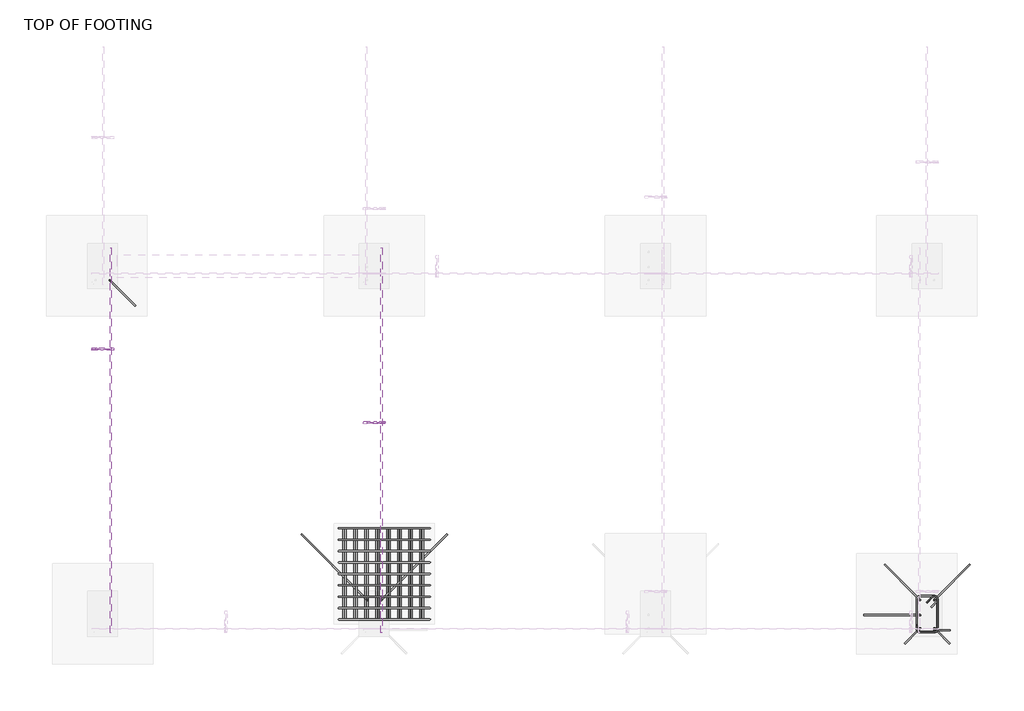
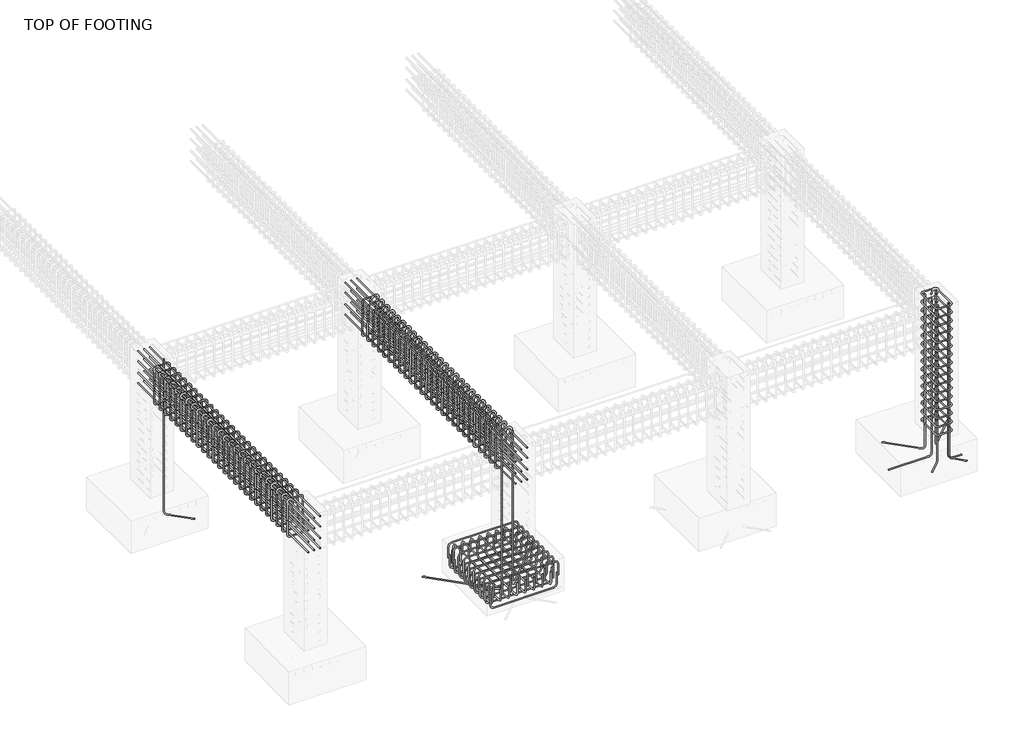
# One storey, part 4 of 14: 24 reinforcing bars.
"""IFC4 building model written with IfcOpenShell, lengths in millimetres."""

from ifc_helpers import new_model, si_unit, point, frame, origin, place, context, project, spatial, polyline, circle_curve, trimmed, segment, composite_curve, source, transform, mapped, element, save
from ifc_brep_helpers import swept_disk

model = new_model("IFC4")

# Units and contexts
model_context = context("Model", 3, world=origin())
ifc_project = project(units=[si_unit("LENGTHUNIT", "METRE", prefix="MILLI")], contexts=[model_context])

# Site, building, storey
site = spatial("IfcSite", under=ifc_project)
building = spatial("IfcBuilding", under=site)
storey = spatial("IfcBuildingStorey", under=building, Name="TOP OF FOOTING", Elevation=-1828.8)

# Reinforcing bars
placement = place(None, origin())
reinforcing_bar_shape = source(origin(), model_context, "Body", "SolidModel", [
    swept_disk(composite_curve([segment(polyline([(-227.457813, 517.7803241, -2035.6107622), (-227.457813, 517.7803241, -2182.9107622)]), True, "CONTINUOUS"), segment(trimmed(circle_curve(frame((-273.807813, 517.7803241, -2182.9107622), z_axis=(0.0, 1.0, 0.0), x_axis=(46.35000000000002, 0.0, 0.0)), 46.35), [point((-227.457813, 517.7803241, -2182.9107622))], [point((-273.807813, 517.7803241, -2229.2607622))], True, "CARTESIAN"), True, "CONTINUOUS"), segment(polyline([(-273.807813, 517.7803241, -2229.2607622), (-1046.4382016, 517.7803241, -2229.2607622)]), True, "CONTINUOUS"), segment(trimmed(circle_curve(frame((-1046.4382016, 517.7803241, -2182.9107622), z_axis=(0.0, 1.0, 0.0), x_axis=(0.0, 0.0, -46.34999999999991)), 46.35), [point((-1046.4382016, 517.7803241, -2229.2607622))], [point((-1092.7882016, 517.7803241, -2182.9107622))], True, "CARTESIAN"), True, "CONTINUOUS"), segment(polyline([(-1092.7882016, 517.7803241, -2182.9107622), (-1092.7882016, 517.7803241, -2035.6107622)]), True, "CONTINUOUS")], self_intersect=False), 6.35),
])
element("IfcReinforcingBar", 1, at=placement, inside=storey, context=model_context, shape_type="MappedRepresentation", body=[
    mapped(reinforcing_bar_shape, transform((0.0, 0.0, 0.0), x_axis=(1.0, 0.0, 0.0), y_axis=(0.0, 1.0, 0.0), z_axis=(0.0, 0.0, 1.0))),
    mapped(reinforcing_bar_shape, transform((0.0, -113.4125, 0.0), x_axis=(1.0, 0.0, 0.0), y_axis=(0.0, 1.0, 0.0), z_axis=(0.0, 0.0, 1.0))),
    mapped(reinforcing_bar_shape, transform((0.0, -226.825, 0.0), x_axis=(1.0, 0.0, 0.0), y_axis=(0.0, 1.0, 0.0), z_axis=(0.0, 0.0, 1.0))),
    mapped(reinforcing_bar_shape, transform((0.0, -340.2375, 0.0), x_axis=(1.0, 0.0, 0.0), y_axis=(0.0, 1.0, 0.0), z_axis=(0.0, 0.0, 1.0))),
    mapped(reinforcing_bar_shape, transform((0.0, -453.65, 0.0), x_axis=(1.0, 0.0, 0.0), y_axis=(0.0, 1.0, 0.0), z_axis=(0.0, 0.0, 1.0))),
    mapped(reinforcing_bar_shape, transform((0.0, -567.0625, 0.0), x_axis=(1.0, 0.0, 0.0), y_axis=(0.0, 1.0, 0.0), z_axis=(0.0, 0.0, 1.0))),
    mapped(reinforcing_bar_shape, transform((0.0, -680.475, 0.0), x_axis=(1.0, 0.0, 0.0), y_axis=(0.0, 1.0, 0.0), z_axis=(0.0, 0.0, 1.0))),
    mapped(reinforcing_bar_shape, transform((0.0, -793.8875, 0.0), x_axis=(1.0, 0.0, 0.0), y_axis=(0.0, 1.0, 0.0), z_axis=(0.0, 0.0, 1.0))),
    mapped(reinforcing_bar_shape, transform((0.0, -907.3, 0.0), x_axis=(1.0, 0.0, 0.0), y_axis=(0.0, 1.0, 0.0), z_axis=(0.0, 0.0, 1.0))),
])
reinforcing_bar_2_shape = source(origin(), model_context, "Body", "SolidModel", [
    swept_disk(composite_curve([segment(polyline([(-1111.0033787, 517.7803241, -2068.991024), (-1111.0033787, 517.7803241, -1921.691024)]), True, "CONTINUOUS"), segment(trimmed(circle_curve(frame((-1064.6533787, 517.7803241, -1921.691024), z_axis=(0.0, 1.0, 0.0), x_axis=(-46.34999999999991, 0.0, 0.0)), 46.35), [point((-1111.0033787, 517.7803241, -1921.691024))], [point((-1064.6533787, 517.7803241, -1875.341024))], True, "CARTESIAN"), True, "CONTINUOUS"), segment(polyline([(-1064.6533787, 517.7803241, -1875.341024), (-250.0533787, 517.7803241, -1875.341024)]), True, "CONTINUOUS"), segment(trimmed(circle_curve(frame((-250.0533787, 517.7803241, -1921.691024), z_axis=(0.0, 1.0, 0.0), x_axis=(0.0, 0.0, 46.34999999999991)), 46.35), [point((-250.0533787, 517.7803241, -1875.341024))], [point((-203.7033787, 517.7803241, -1921.691024))], True, "CARTESIAN"), True, "CONTINUOUS"), segment(polyline([(-203.7033787, 517.7803241, -1921.691024), (-203.7033787, 517.7803241, -2068.991024)]), True, "CONTINUOUS")], self_intersect=False), 6.35),
])
element("IfcReinforcingBar", 2, at=placement, inside=storey, context=model_context, shape_type="MappedRepresentation", body=[
    mapped(reinforcing_bar_2_shape, transform((0.0, 0.0, 0.0), x_axis=(1.0, 0.0, 0.0), y_axis=(0.0, 1.0, 0.0), z_axis=(0.0, 0.0, 1.0))),
    mapped(reinforcing_bar_2_shape, transform((0.0, -113.4125, 0.0), x_axis=(1.0, 0.0, 0.0), y_axis=(0.0, 1.0, 0.0), z_axis=(0.0, 0.0, 1.0))),
    mapped(reinforcing_bar_2_shape, transform((0.0, -226.825, 0.0), x_axis=(1.0, 0.0, 0.0), y_axis=(0.0, 1.0, 0.0), z_axis=(0.0, 0.0, 1.0))),
    mapped(reinforcing_bar_2_shape, transform((0.0, -340.2375, 0.0), x_axis=(1.0, 0.0, 0.0), y_axis=(0.0, 1.0, 0.0), z_axis=(0.0, 0.0, 1.0))),
    mapped(reinforcing_bar_2_shape, transform((0.0, -453.65, 0.0), x_axis=(1.0, 0.0, 0.0), y_axis=(0.0, 1.0, 0.0), z_axis=(0.0, 0.0, 1.0))),
    mapped(reinforcing_bar_2_shape, transform((0.0, -567.0625, 0.0), x_axis=(1.0, 0.0, 0.0), y_axis=(0.0, 1.0, 0.0), z_axis=(0.0, 0.0, 1.0))),
    mapped(reinforcing_bar_2_shape, transform((0.0, -680.475, 0.0), x_axis=(1.0, 0.0, 0.0), y_axis=(0.0, 1.0, 0.0), z_axis=(0.0, 0.0, 1.0))),
    mapped(reinforcing_bar_2_shape, transform((0.0, -793.8875, 0.0), x_axis=(1.0, 0.0, 0.0), y_axis=(0.0, 1.0, 0.0), z_axis=(0.0, 0.0, 1.0))),
    mapped(reinforcing_bar_2_shape, transform((0.0, -907.3, 0.0), x_axis=(1.0, 0.0, 0.0), y_axis=(0.0, 1.0, 0.0), z_axis=(0.0, 0.0, 1.0))),
])
reinforcing_bar_3_shape = source(origin(), model_context, "Body", "SolidModel", [
    swept_disk(composite_curve([segment(polyline([(-273.4932847, 517.7803241, -2085.4684936), (-273.4932847, 517.7803241, -1938.1684936)]), True, "CONTINUOUS"), segment(trimmed(circle_curve(frame((-273.4932847, 471.4303241, -1938.1684936), z_axis=(1.0, 0.0, 0.0), x_axis=(0.0, 46.35000000000002, 0.0)), 46.35), [point((-273.4932847, 517.7803241, -1938.1684936))], [point((-273.4932847, 471.4303241, -1891.8184936))], True, "CARTESIAN"), True, "CONTINUOUS"), segment(polyline([(-273.4932847, 471.4303241, -1891.8184936), (-273.4932847, -343.1696759, -1891.8184936)]), True, "CONTINUOUS"), segment(trimmed(circle_curve(frame((-273.4932847, -343.1696759, -1938.1684936), z_axis=(1.0, 0.0, 0.0), x_axis=(0.0, 0.0, 46.34999999999991)), 46.35), [point((-273.4932847, -343.1696759, -1891.8184936))], [point((-273.4932847, -389.5196759, -1938.1684936))], True, "CARTESIAN"), True, "CONTINUOUS"), segment(polyline([(-273.4932847, -389.5196759, -1938.1684936), (-273.4932847, -389.5196759, -2085.4684936)]), True, "CONTINUOUS")], self_intersect=False), 6.35),
])
element("IfcReinforcingBar", 3, at=placement, inside=storey, context=model_context, shape_type="MappedRepresentation", body=[
    mapped(reinforcing_bar_3_shape, transform((0.0, 0.0, 0.0), x_axis=(1.0, 0.0, 0.0), y_axis=(0.0, 1.0, 0.0), z_axis=(0.0, 0.0, 1.0))),
    mapped(reinforcing_bar_3_shape, transform((-110.0713853, 0.0, 0.0), x_axis=(1.0, 0.0, 0.0), y_axis=(0.0, 1.0, 0.0), z_axis=(0.0, 0.0, 1.0))),
    mapped(reinforcing_bar_3_shape, transform((-220.1427706, 0.0, 0.0), x_axis=(1.0, 0.0, 0.0), y_axis=(0.0, 1.0, 0.0), z_axis=(0.0, 0.0, 1.0))),
    mapped(reinforcing_bar_3_shape, transform((-330.2141558, 0.0, 0.0), x_axis=(1.0, 0.0, 0.0), y_axis=(0.0, 1.0, 0.0), z_axis=(0.0, 0.0, 1.0))),
    mapped(reinforcing_bar_3_shape, transform((-440.2855411, 0.0, 0.0), x_axis=(1.0, 0.0, 0.0), y_axis=(0.0, 1.0, 0.0), z_axis=(0.0, 0.0, 1.0))),
    mapped(reinforcing_bar_3_shape, transform((-550.3569264, 0.0, 0.0), x_axis=(1.0, 0.0, 0.0), y_axis=(0.0, 1.0, 0.0), z_axis=(0.0, 0.0, 1.0))),
    mapped(reinforcing_bar_3_shape, transform((-660.4283117, 0.0, 0.0), x_axis=(1.0, 0.0, 0.0), y_axis=(0.0, 1.0, 0.0), z_axis=(0.0, 0.0, 1.0))),
    mapped(reinforcing_bar_3_shape, transform((-770.4996969, 0.0, 0.0), x_axis=(1.0, 0.0, 0.0), y_axis=(0.0, 1.0, 0.0), z_axis=(0.0, 0.0, 1.0))),
])
reinforcing_bar_4_shape = source(origin(), model_context, "Body", "SolidModel", [
    swept_disk(composite_curve([segment(polyline([(-1062.3533787, 517.7803241, -1990.15), (-1062.3533787, 517.7803241, -2137.45)]), True, "CONTINUOUS"), segment(trimmed(circle_curve(frame((-1062.3533787, 471.4303241, -2137.45), z_axis=(-1.0, 0.0, 0.0), x_axis=(0.0, 46.35000000000002, 0.0)), 46.35), [point((-1062.3533787, 517.7803241, -2137.45))], [point((-1062.3533787, 471.4303241, -2183.8))], True, "CARTESIAN"), True, "CONTINUOUS"), segment(polyline([(-1062.3533787, 471.4303241, -2183.8), (-1062.3533787, -343.1696759, -2183.8)]), True, "CONTINUOUS"), segment(trimmed(circle_curve(frame((-1062.3533787, -343.1696759, -2137.45), z_axis=(-1.0, 0.0, 0.0), x_axis=(0.0, 0.0, -46.350000000000364)), 46.35), [point((-1062.3533787, -343.1696759, -2183.8))], [point((-1062.3533787, -389.5196759, -2137.45))], True, "CARTESIAN"), True, "CONTINUOUS"), segment(polyline([(-1062.3533787, -389.5196759, -2137.45), (-1062.3533787, -389.5196759, -1990.15)]), True, "CONTINUOUS")], self_intersect=False), 6.35),
])
element("IfcReinforcingBar", 4, at=placement, inside=storey, context=model_context, shape_type="MappedRepresentation", body=[
    mapped(reinforcing_bar_4_shape, transform((0.0, 0.0, 0.0), x_axis=(1.0, 0.0, 0.0), y_axis=(0.0, 1.0, 0.0), z_axis=(0.0, 0.0, 1.0))),
    mapped(reinforcing_bar_4_shape, transform((108.7810905, 0.0, 0.0), x_axis=(1.0, 0.0, 0.0), y_axis=(0.0, 1.0, 0.0), z_axis=(0.0, 0.0, 1.0))),
    mapped(reinforcing_bar_4_shape, transform((217.5621811, 0.0, 0.0), x_axis=(1.0, 0.0, 0.0), y_axis=(0.0, 1.0, 0.0), z_axis=(0.0, 0.0, 1.0))),
    mapped(reinforcing_bar_4_shape, transform((326.3432716, 0.0, 0.0), x_axis=(1.0, 0.0, 0.0), y_axis=(0.0, 1.0, 0.0), z_axis=(0.0, 0.0, 1.0))),
    mapped(reinforcing_bar_4_shape, transform((435.1243621, 0.0, 0.0), x_axis=(1.0, 0.0, 0.0), y_axis=(0.0, 1.0, 0.0), z_axis=(0.0, 0.0, 1.0))),
    mapped(reinforcing_bar_4_shape, transform((543.9054526, 0.0, 0.0), x_axis=(1.0, 0.0, 0.0), y_axis=(0.0, 1.0, 0.0), z_axis=(0.0, 0.0, 1.0))),
    mapped(reinforcing_bar_4_shape, transform((652.6865432, 0.0, 0.0), x_axis=(1.0, 0.0, 0.0), y_axis=(0.0, 1.0, 0.0), z_axis=(0.0, 0.0, 1.0))),
    mapped(reinforcing_bar_4_shape, transform((761.4676337, 0.0, 0.0), x_axis=(1.0, 0.0, 0.0), y_axis=(0.0, 1.0, 0.0), z_axis=(0.0, 0.0, 1.0))),
])
element("IfcReinforcingBar", 5, at=placement, inside=storey, context=model_context, shape_type="SolidModel", body=[
    swept_disk(composite_curve([segment(polyline([(-3386.7020371, 2984.1707812, -40.0), (-3386.7020371, 2984.1707812, -2122.4113862)]), True, "CONTINUOUS"), segment(trimmed(circle_curve(frame((-3353.9276378, 2951.3963819, -2122.4113862), z_axis=(-0.7071067811865441, -0.707106781186551, 0.0), x_axis=(-32.774399299999914, 32.774399299999914, 0.0)), 46.35), [point((-3386.7020371, 2984.1707812, -2122.4113862))], [point((-3353.9276378, 2951.3963819, -2168.7613862))], True, "CARTESIAN"), True, "CONTINUOUS"), segment(polyline([(-3353.9276378, 2951.3963819, -2168.7613862), (-3133.2315258, 2730.7002699, -2168.7613862)]), True, "CONTINUOUS")], self_intersect=False), 6.35),
])
element("IfcReinforcingBar", 6, at=placement, inside=storey, context=model_context, shape_type="SolidModel", body=[
    swept_disk(composite_curve([segment(polyline([(-686.7020371, -195.7905774, -40.0), (-686.7020371, -195.7905774, -2122.4113862)]), True, "CONTINUOUS"), segment(trimmed(circle_curve(frame((-653.9276378, -163.0161781, -2122.4113862), z_axis=(0.7071067811865235, -0.7071067811865717, 0.0), x_axis=(-32.77439930000003, -32.7743993, 0.0)), 46.35), [point((-686.7020371, -195.7905774, -2122.4113862))], [point((-653.9276378, -163.0161781, -2168.7613862))], True, "CARTESIAN"), True, "CONTINUOUS"), segment(polyline([(-653.9276378, -163.0161781, -2168.7613862), (-33.2315258, 457.6799339, -2168.7613862)]), True, "CONTINUOUS")], self_intersect=False), 6.35),
])
element("IfcReinforcingBar", 7, at=placement, inside=storey, context=model_context, shape_type="SolidModel", body=[
    swept_disk(composite_curve([segment(polyline([(-828.0047203, -195.7905774, -40.0), (-828.0047203, -195.7905774, -2122.4113862)]), True, "CONTINUOUS"), segment(trimmed(circle_curve(frame((-860.7791196, -163.0161781, -2122.4113862), z_axis=(0.7071067811865548, 0.7071067811865404, 0.0), x_axis=(32.774399299999914, -32.7743993, 0.0)), 46.35), [point((-828.0047203, -195.7905774, -2122.4113862))], [point((-860.7791196, -163.0161781, -2168.7613862))], True, "CARTESIAN"), True, "CONTINUOUS"), segment(polyline([(-860.7791196, -163.0161781, -2168.7613862), (-1481.4752316, 457.6799339, -2168.7613862)]), True, "CONTINUOUS")], self_intersect=False), 6.35),
])
reinforcing_bar_5_shape = source(origin(), model_context, "Body", "SolidModel", [
    swept_disk(composite_curve([segment(polyline([(4737.0352608, -222.1454413, -46.35), (4792.7788237, -166.4018783, -46.35)]), True, "CONTINUOUS"), segment(trimmed(circle_curve(frame((4814.9466213, -188.5696759, -46.35), z_axis=(0.0, 0.0, -1.0), x_axis=(-22.167797599999176, 22.1677976, 0.0)), 31.35), [point((4792.7788237, -166.4018783, -46.35))], [point((4846.2966213, -188.5696759, -46.35))], True, "CARTESIAN"), True, "CONTINUOUS"), segment(polyline([(4846.2966213, -188.5696759, -46.35), (4846.2966213, -483.1696759, -46.35)]), True, "CONTINUOUS"), segment(trimmed(circle_curve(frame((4814.9466213, -483.1696759, -46.35), z_axis=(0.0, 0.0, -1.0), x_axis=(31.350000000000364, 0.0, 0.0)), 31.35), [point((4846.2966213, -483.1696759, -46.35))], [point((4814.9466213, -514.5196759, -46.35))], True, "CARTESIAN"), True, "CONTINUOUS"), segment(polyline([(4814.9466213, -514.5196759, -46.35), (4670.3466213, -514.5196759, -46.35)]), True, "CONTINUOUS"), segment(trimmed(circle_curve(frame((4670.3466213, -483.189461, -45.2363875), z_axis=(0.0, 0.03552192833448213, -0.9993688971583016), x_axis=(0.0, -31.330214900000044, -1.1136125000000021)), 31.35), [point((4670.3466213, -514.5196759, -46.35))], [point((4638.9966213, -483.189461, -45.2363875))], True, "CARTESIAN"), True, "CONTINUOUS"), segment(polyline([(4638.9966213, -483.189461, -45.2363875), (4638.9966213, -188.5498908, -34.7636125)]), True, "CONTINUOUS"), segment(trimmed(circle_curve(frame((4670.3466213, -188.5498908, -34.7636125), z_axis=(0.0, 0.03552192833448213, -0.9993688971583016), x_axis=(-31.350000000000364, 0.0, 0.0)), 31.35), [point((4638.9966213, -188.5498908, -34.7636125))], [point((4670.3466213, -157.2196759, -33.65))], True, "CARTESIAN"), True, "CONTINUOUS"), segment(polyline([(4670.3466213, -157.2196759, -33.65), (4814.9466213, -157.2196759, -33.65)]), True, "CONTINUOUS"), segment(trimmed(circle_curve(frame((4814.9466213, -188.5696759, -33.65), z_axis=(0.0, 0.0, -1.0), x_axis=(0.0, 31.349999999999994, 0.0)), 31.35), [point((4814.9466213, -157.2196759, -33.65))], [point((4837.1144189, -210.7374735, -33.65))], True, "CARTESIAN"), True, "CONTINUOUS"), segment(polyline([(4837.1144189, -210.7374735, -33.65), (4781.3708559, -266.4810364, -33.65)]), True, "CONTINUOUS")], self_intersect=False), 6.35),
])
element("IfcReinforcingBar", 8, at=placement, inside=storey, context=model_context, shape_type="MappedRepresentation", body=[
    mapped(reinforcing_bar_5_shape, transform((0.0, 0.0, 0.0), x_axis=(1.0, 0.0, 0.0), y_axis=(0.0, 1.0, 0.0), z_axis=(0.0, 0.0, 1.0))),
    mapped(reinforcing_bar_5_shape, transform((0.0, 0.0, -115.74), x_axis=(1.0, 0.0, 0.0), y_axis=(0.0, 1.0, 0.0), z_axis=(0.0, 0.0, 1.0))),
    mapped(reinforcing_bar_5_shape, transform((0.0, 0.0, -231.48), x_axis=(1.0, 0.0, 0.0), y_axis=(0.0, 1.0, 0.0), z_axis=(0.0, 0.0, 1.0))),
    mapped(reinforcing_bar_5_shape, transform((0.0, 0.0, -347.22), x_axis=(1.0, 0.0, 0.0), y_axis=(0.0, 1.0, 0.0), z_axis=(0.0, 0.0, 1.0))),
    mapped(reinforcing_bar_5_shape, transform((0.0, 0.0, -462.96), x_axis=(1.0, 0.0, 0.0), y_axis=(0.0, 1.0, 0.0), z_axis=(0.0, 0.0, 1.0))),
    mapped(reinforcing_bar_5_shape, transform((0.0, 0.0, -578.7), x_axis=(1.0, 0.0, 0.0), y_axis=(0.0, 1.0, 0.0), z_axis=(0.0, 0.0, 1.0))),
    mapped(reinforcing_bar_5_shape, transform((0.0, 0.0, -694.44), x_axis=(1.0, 0.0, 0.0), y_axis=(0.0, 1.0, 0.0), z_axis=(0.0, 0.0, 1.0))),
    mapped(reinforcing_bar_5_shape, transform((0.0, 0.0, -810.18), x_axis=(1.0, 0.0, 0.0), y_axis=(0.0, 1.0, 0.0), z_axis=(0.0, 0.0, 1.0))),
    mapped(reinforcing_bar_5_shape, transform((0.0, 0.0, -925.92), x_axis=(1.0, 0.0, 0.0), y_axis=(0.0, 1.0, 0.0), z_axis=(0.0, 0.0, 1.0))),
    mapped(reinforcing_bar_5_shape, transform((0.0, 0.0, -1041.66), x_axis=(1.0, 0.0, 0.0), y_axis=(0.0, 1.0, 0.0), z_axis=(0.0, 0.0, 1.0))),
    mapped(reinforcing_bar_5_shape, transform((0.0, 0.0, -1157.4), x_axis=(1.0, 0.0, 0.0), y_axis=(0.0, 1.0, 0.0), z_axis=(0.0, 0.0, 1.0))),
    mapped(reinforcing_bar_5_shape, transform((0.0, 0.0, -1273.14), x_axis=(1.0, 0.0, 0.0), y_axis=(0.0, 1.0, 0.0), z_axis=(0.0, 0.0, 1.0))),
    mapped(reinforcing_bar_5_shape, transform((0.0, 0.0, -1388.88), x_axis=(1.0, 0.0, 0.0), y_axis=(0.0, 1.0, 0.0), z_axis=(0.0, 0.0, 1.0))),
    mapped(reinforcing_bar_5_shape, transform((0.0, 0.0, -1504.62), x_axis=(1.0, 0.0, 0.0), y_axis=(0.0, 1.0, 0.0), z_axis=(0.0, 0.0, 1.0))),
    mapped(reinforcing_bar_5_shape, transform((0.0, 0.0, -1620.36), x_axis=(1.0, 0.0, 0.0), y_axis=(0.0, 1.0, 0.0), z_axis=(0.0, 0.0, 1.0))),
    mapped(reinforcing_bar_5_shape, transform((0.0, 0.0, -1736.1), x_axis=(1.0, 0.0, 0.0), y_axis=(0.0, 1.0, 0.0), z_axis=(0.0, 0.0, 1.0))),
])
element("IfcReinforcingBar", 9, at=placement, inside=storey, context=model_context, shape_type="SolidModel", body=[
    swept_disk(composite_curve([segment(polyline([(4813.2979629, -495.9487744, -40.0), (4813.2979629, -495.9487744, -2122.4113862)]), True, "CONTINUOUS"), segment(trimmed(circle_curve(frame((4859.6479629, -495.9487744, -2122.4113862), z_axis=(0.0, -1.0, 0.0), x_axis=(-46.349999999999454, 0.0, 0.0)), 46.35), [point((4813.2979629, -495.9487744, -2122.4113862))], [point((4859.6479629, -495.9487744, -2168.7613862))], True, "CARTESIAN"), True, "CONTINUOUS"), segment(polyline([(4859.6479629, -495.9487744, -2168.7613862), (4971.7593977, -495.9487744, -2168.7613862)]), True, "CONTINUOUS")], self_intersect=False), 6.35),
])
element("IfcReinforcingBar", 10, at=placement, inside=storey, context=model_context, shape_type="SolidModel", body=[
    swept_disk(composite_curve([segment(polyline([(4813.2979629, -475.9487744, -40.0), (4813.2979629, -475.9487744, -2122.4113862)]), True, "CONTINUOUS"), segment(trimmed(circle_curve(frame((4846.0723622, -508.7231737, -2122.4113862), z_axis=(-0.7071067811865441, -0.707106781186551, 0.0), x_axis=(-32.77439929999946, 32.77439930000003, 0.0)), 46.35), [point((4813.2979629, -475.9487744, -2122.4113862))], [point((4846.0723622, -508.7231737, -2168.7613862))], True, "CARTESIAN"), True, "CONTINUOUS"), segment(polyline([(4846.0723622, -508.7231737, -2168.7613862), (4966.7684742, -629.4192858, -2168.7613862)]), True, "CONTINUOUS")], self_intersect=False), 6.35),
])
element("IfcReinforcingBar", 11, at=placement, inside=storey, context=model_context, shape_type="SolidModel", body=[
    swept_disk(composite_curve([segment(polyline([(4671.9952797, -475.9487744, -40.0), (4671.9952797, -475.9487744, -2122.4113862)]), True, "CONTINUOUS"), segment(trimmed(circle_curve(frame((4639.2208804, -508.7231737, -2122.4113862), z_axis=(-0.7071067811865341, 0.707106781186561, 0.0), x_axis=(32.77439929999946, 32.77439930000003, 0.0)), 46.35), [point((4671.9952797, -475.9487744, -2122.4113862))], [point((4639.2208804, -508.7231737, -2168.7613862))], True, "CARTESIAN"), True, "CONTINUOUS"), segment(polyline([(4639.2208804, -508.7231737, -2168.7613862), (4518.5247684, -629.4192858, -2168.7613862)]), True, "CONTINUOUS")], self_intersect=False), 6.35),
])
element("IfcReinforcingBar", 12, at=placement, inside=storey, context=model_context, shape_type="SolidModel", body=[
    swept_disk(composite_curve([segment(polyline([(4813.2979629, -195.7905774, -40.0), (4813.2979629, -195.7905774, -2122.4113862)]), True, "CONTINUOUS"), segment(trimmed(circle_curve(frame((4846.0723622, -163.0161781, -2122.4113862), z_axis=(0.7071067811865235, -0.7071067811865717, 0.0), x_axis=(-32.77439929999946, -32.7743993, 0.0)), 46.35), [point((4813.2979629, -195.7905774, -2122.4113862))], [point((4846.0723622, -163.0161781, -2168.7613862))], True, "CARTESIAN"), True, "CONTINUOUS"), segment(polyline([(4846.0723622, -163.0161781, -2168.7613862), (5166.7684742, 157.6799339, -2168.7613862)]), True, "CONTINUOUS")], self_intersect=False), 6.35),
])
element("IfcReinforcingBar", 13, at=placement, inside=storey, context=model_context, shape_type="SolidModel", body=[
    swept_disk(composite_curve([segment(polyline([(4671.9952797, -195.7905774, -40.0), (4671.9952797, -195.7905774, -2122.4113862)]), True, "CONTINUOUS"), segment(trimmed(circle_curve(frame((4639.2208804, -163.0161781, -2122.4113862), z_axis=(0.7071067811865548, 0.7071067811865404, 0.0), x_axis=(32.77439929999946, -32.7743993, 0.0)), 46.35), [point((4671.9952797, -195.7905774, -2122.4113862))], [point((4639.2208804, -163.0161781, -2168.7613862))], True, "CARTESIAN"), True, "CONTINUOUS"), segment(polyline([(4639.2208804, -163.0161781, -2168.7613862), (4318.5247684, 157.6799339, -2168.7613862)]), True, "CONTINUOUS")], self_intersect=False), 6.35),
])
element("IfcReinforcingBar", 14, at=placement, inside=storey, context=model_context, shape_type="SolidModel", body=[
    swept_disk(composite_curve([segment(polyline([(4671.9952797, -345.9487744, -40.0), (4671.9952797, -345.9487744, -2122.4113862)]), True, "CONTINUOUS"), segment(trimmed(circle_curve(frame((4625.6452797, -345.9487744, -2122.4113862), z_axis=(0.0, 1.0, 0.0), x_axis=(46.349999999999454, 0.0, 0.0)), 46.35), [point((4671.9952797, -345.9487744, -2122.4113862))], [point((4625.6452797, -345.9487744, -2168.7613862))], True, "CARTESIAN"), True, "CONTINUOUS"), segment(polyline([(4625.6452797, -345.9487744, -2168.7613862), (4113.5338449, -345.9487744, -2168.7613862)]), True, "CONTINUOUS")], self_intersect=False), 6.35),
])
reinforcing_bar_6_shape = source(origin(), model_context, "Body", "SolidModel", [
    swept_disk(composite_curve([segment(polyline([(-762.9647392, -104.5196759, -111.2757654), (-707.2211763, -104.5196759, -55.5322024)]), True, "CONTINUOUS"), segment(trimmed(circle_curve(frame((-685.0533787, -104.5196759, -77.7), z_axis=(0.0, 1.0, 0.0), x_axis=(-22.16779759999997, 0.0, 22.1677976)), 31.35), [point((-707.2211763, -104.5196759, -55.5322024))], [point((-653.7033787, -104.5196759, -77.7))], True, "CARTESIAN"), True, "CONTINUOUS"), segment(polyline([(-653.7033787, -104.5196759, -77.7), (-653.7033787, -104.5196759, -522.3)]), True, "CONTINUOUS"), segment(trimmed(circle_curve(frame((-685.0533787, -104.5196759, -522.3), z_axis=(0.0, 1.0, 0.0), x_axis=(31.350000000000023, 0.0, 0.0)), 31.35), [point((-653.7033787, -104.5196759, -522.3))], [point((-685.0533787, -104.5196759, -553.65))], True, "CARTESIAN"), True, "CONTINUOUS"), segment(polyline([(-685.0533787, -104.5196759, -553.65), (-829.6533787, -104.5196759, -553.65)]), True, "CONTINUOUS"), segment(trimmed(circle_curve(frame((-829.6533787, -105.3042615, -522.3098193), z_axis=(0.0, 0.9996867842138424, 0.025026655153786322), x_axis=(0.0, 0.7845855999999998, -31.34018070000002)), 31.35), [point((-829.6533787, -104.5196759, -553.65))], [point((-861.0033787, -105.3042615, -522.3098193))], True, "CARTESIAN"), True, "CONTINUOUS"), segment(polyline([(-861.0033787, -105.3042615, -522.3098193), (-861.0033787, -116.4350903, -77.6901807)]), True, "CONTINUOUS"), segment(trimmed(circle_curve(frame((-829.6533787, -116.4350903, -77.6901807), z_axis=(0.0, 0.9996867842138424, 0.025026655153786322), x_axis=(-31.350000000000023, 0.0, 0.0)), 31.35), [point((-861.0033787, -116.4350903, -77.6901807))], [point((-829.6533787, -117.2196759, -46.35))], True, "CARTESIAN"), True, "CONTINUOUS"), segment(polyline([(-829.6533787, -117.2196759, -46.35), (-685.0533787, -117.2196759, -46.35)]), True, "CONTINUOUS"), segment(trimmed(circle_curve(frame((-685.0533787, -117.2196759, -77.7), z_axis=(0.0, 1.0, 0.0), x_axis=(0.0, 0.0, 31.35)), 31.35), [point((-685.0533787, -117.2196759, -46.35))], [point((-662.8855811, -117.2196759, -99.8677976))], True, "CARTESIAN"), True, "CONTINUOUS"), segment(polyline([(-662.8855811, -117.2196759, -99.8677976), (-718.6291441, -117.2196759, -155.6113605)]), True, "CONTINUOUS")], self_intersect=False), 6.35),
])
element("IfcReinforcingBar", 15, at=placement, inside=storey, context=model_context, shape_type="MappedRepresentation", body=[
    mapped(reinforcing_bar_6_shape, transform((0.0, 0.0, 0.0), x_axis=(1.0, 0.0, 0.0), y_axis=(0.0, 1.0, 0.0), z_axis=(0.0, 0.0, 1.0))),
    mapped(reinforcing_bar_6_shape, transform((0.0, 119.8967822, 0.0), x_axis=(1.0, 0.0, 0.0), y_axis=(0.0, 1.0, 0.0), z_axis=(0.0, 0.0, 1.0))),
    mapped(reinforcing_bar_6_shape, transform((0.0, 239.7935645, 0.0), x_axis=(1.0, 0.0, 0.0), y_axis=(0.0, 1.0, 0.0), z_axis=(0.0, 0.0, 1.0))),
    mapped(reinforcing_bar_6_shape, transform((0.0, 359.6903467, 0.0), x_axis=(1.0, 0.0, 0.0), y_axis=(0.0, 1.0, 0.0), z_axis=(0.0, 0.0, 1.0))),
    mapped(reinforcing_bar_6_shape, transform((0.0, 479.5871289, 0.0), x_axis=(1.0, 0.0, 0.0), y_axis=(0.0, 1.0, 0.0), z_axis=(0.0, 0.0, 1.0))),
    mapped(reinforcing_bar_6_shape, transform((0.0, 599.4839111, 0.0), x_axis=(1.0, 0.0, 0.0), y_axis=(0.0, 1.0, 0.0), z_axis=(0.0, 0.0, 1.0))),
    mapped(reinforcing_bar_6_shape, transform((0.0, 719.3806934, 0.0), x_axis=(1.0, 0.0, 0.0), y_axis=(0.0, 1.0, 0.0), z_axis=(0.0, 0.0, 1.0))),
    mapped(reinforcing_bar_6_shape, transform((0.0, 839.2774756, 0.0), x_axis=(1.0, 0.0, 0.0), y_axis=(0.0, 1.0, 0.0), z_axis=(0.0, 0.0, 1.0))),
    mapped(reinforcing_bar_6_shape, transform((0.0, 959.1742578, 0.0), x_axis=(1.0, 0.0, 0.0), y_axis=(0.0, 1.0, 0.0), z_axis=(0.0, 0.0, 1.0))),
    mapped(reinforcing_bar_6_shape, transform((0.0, 1079.07104, 0.0), x_axis=(1.0, 0.0, 0.0), y_axis=(0.0, 1.0, 0.0), z_axis=(0.0, 0.0, 1.0))),
    mapped(reinforcing_bar_6_shape, transform((0.0, 1198.9678223, 0.0), x_axis=(1.0, 0.0, 0.0), y_axis=(0.0, 1.0, 0.0), z_axis=(0.0, 0.0, 1.0))),
    mapped(reinforcing_bar_6_shape, transform((0.0, 1318.8646045, 0.0), x_axis=(1.0, 0.0, 0.0), y_axis=(0.0, 1.0, 0.0), z_axis=(0.0, 0.0, 1.0))),
    mapped(reinforcing_bar_6_shape, transform((0.0, 1438.7613867, 0.0), x_axis=(1.0, 0.0, 0.0), y_axis=(0.0, 1.0, 0.0), z_axis=(0.0, 0.0, 1.0))),
    mapped(reinforcing_bar_6_shape, transform((0.0, 1558.658169, 0.0), x_axis=(1.0, 0.0, 0.0), y_axis=(0.0, 1.0, 0.0), z_axis=(0.0, 0.0, 1.0))),
    mapped(reinforcing_bar_6_shape, transform((0.0, 1678.5549512, 0.0), x_axis=(1.0, 0.0, 0.0), y_axis=(0.0, 1.0, 0.0), z_axis=(0.0, 0.0, 1.0))),
    mapped(reinforcing_bar_6_shape, transform((0.0, 1798.4517334, 0.0), x_axis=(1.0, 0.0, 0.0), y_axis=(0.0, 1.0, 0.0), z_axis=(0.0, 0.0, 1.0))),
    mapped(reinforcing_bar_6_shape, transform((0.0, 1918.3485156, 0.0), x_axis=(1.0, 0.0, 0.0), y_axis=(0.0, 1.0, 0.0), z_axis=(0.0, 0.0, 1.0))),
    mapped(reinforcing_bar_6_shape, transform((0.0, 2038.2452979, 0.0), x_axis=(1.0, 0.0, 0.0), y_axis=(0.0, 1.0, 0.0), z_axis=(0.0, 0.0, 1.0))),
    mapped(reinforcing_bar_6_shape, transform((0.0, 2158.1420801, 0.0), x_axis=(1.0, 0.0, 0.0), y_axis=(0.0, 1.0, 0.0), z_axis=(0.0, 0.0, 1.0))),
    mapped(reinforcing_bar_6_shape, transform((0.0, 2278.0388623, 0.0), x_axis=(1.0, 0.0, 0.0), y_axis=(0.0, 1.0, 0.0), z_axis=(0.0, 0.0, 1.0))),
    mapped(reinforcing_bar_6_shape, transform((0.0, 2397.9356445, 0.0), x_axis=(1.0, 0.0, 0.0), y_axis=(0.0, 1.0, 0.0), z_axis=(0.0, 0.0, 1.0))),
    mapped(reinforcing_bar_6_shape, transform((0.0, 2517.8324268, 0.0), x_axis=(1.0, 0.0, 0.0), y_axis=(0.0, 1.0, 0.0), z_axis=(0.0, 0.0, 1.0))),
    mapped(reinforcing_bar_6_shape, transform((0.0, 2637.729209, 0.0), x_axis=(1.0, 0.0, 0.0), y_axis=(0.0, 1.0, 0.0), z_axis=(0.0, 0.0, 1.0))),
    mapped(reinforcing_bar_6_shape, transform((0.0, 2757.6259912, 0.0), x_axis=(1.0, 0.0, 0.0), y_axis=(0.0, 1.0, 0.0), z_axis=(0.0, 0.0, 1.0))),
    mapped(reinforcing_bar_6_shape, transform((0.0, 2877.5227734, 0.0), x_axis=(1.0, 0.0, 0.0), y_axis=(0.0, 1.0, 0.0), z_axis=(0.0, 0.0, 1.0))),
    mapped(reinforcing_bar_6_shape, transform((0.0, 2997.4195557, 0.0), x_axis=(1.0, 0.0, 0.0), y_axis=(0.0, 1.0, 0.0), z_axis=(0.0, 0.0, 1.0))),
])
reinforcing_bar_7_shape = source(origin(), model_context, "Body", "SolidModel", [
    swept_disk(composite_curve([segment(polyline([(-837.0996321, -520.8696759, -77.7), (-837.0996321, 3309.2498798, -77.7)]), True, "CONTINUOUS")], self_intersect=False), 6.35),
])
element("IfcReinforcingBar", 16, at=placement, inside=storey, context=model_context, shape_type="MappedRepresentation", body=[
    mapped(reinforcing_bar_7_shape, transform((0.0, 0.0, 0.0), x_axis=(1.0, 0.0, 0.0), y_axis=(0.0, 1.0, 0.0), z_axis=(0.0, 0.0, 1.0))),
    mapped(reinforcing_bar_7_shape, transform((76.0102945, 0.0, 0.0), x_axis=(1.0, 0.0, 0.0), y_axis=(0.0, 1.0, 0.0), z_axis=(0.0, 0.0, 1.0))),
    mapped(reinforcing_bar_7_shape, transform((152.0205889, 0.0, 0.0), x_axis=(1.0, 0.0, 0.0), y_axis=(0.0, 1.0, 0.0), z_axis=(0.0, 0.0, 1.0))),
])
reinforcing_bar_8_shape = source(origin(), model_context, "Body", "SolidModel", [
    swept_disk(composite_curve([segment(polyline([(-837.0996321, -520.8696759, -517.7), (-837.0996321, 3309.2498798, -517.7)]), True, "CONTINUOUS")], self_intersect=False), 6.35),
])
element("IfcReinforcingBar", 17, at=placement, inside=storey, context=model_context, shape_type="MappedRepresentation", body=[
    mapped(reinforcing_bar_8_shape, transform((0.0, 0.0, 0.0), x_axis=(1.0, 0.0, 0.0), y_axis=(0.0, 1.0, 0.0), z_axis=(0.0, 0.0, 1.0))),
    mapped(reinforcing_bar_8_shape, transform((76.0102945, 0.0, 0.0), x_axis=(1.0, 0.0, 0.0), y_axis=(0.0, 1.0, 0.0), z_axis=(0.0, 0.0, 1.0))),
    mapped(reinforcing_bar_8_shape, transform((152.0205889, 0.0, 0.0), x_axis=(1.0, 0.0, 0.0), y_axis=(0.0, 1.0, 0.0), z_axis=(0.0, 0.0, 1.0))),
])
reinforcing_bar_9_shape = source(origin(), model_context, "Body", "SolidModel", [
    swept_disk(composite_curve([segment(polyline([(-837.0996321, -520.8696759, -377.7), (-837.0996321, 3309.2498798, -377.7)]), True, "CONTINUOUS")], self_intersect=False), 6.35),
])
element("IfcReinforcingBar", 18, at=placement, inside=storey, context=model_context, shape_type="MappedRepresentation", body=[
    mapped(reinforcing_bar_9_shape, transform((0.0, 0.0, 0.0), x_axis=(1.0, 0.0, 0.0), y_axis=(0.0, 1.0, 0.0), z_axis=(0.0, 0.0, 1.0))),
    mapped(reinforcing_bar_9_shape, transform((76.0102945, 0.0, 0.0), x_axis=(1.0, 0.0, 0.0), y_axis=(0.0, 1.0, 0.0), z_axis=(0.0, 0.0, 1.0))),
    mapped(reinforcing_bar_9_shape, transform((152.0205889, 0.0, 0.0), x_axis=(1.0, 0.0, 0.0), y_axis=(0.0, 1.0, 0.0), z_axis=(0.0, 0.0, 1.0))),
])
reinforcing_bar_10_shape = source(origin(), model_context, "Body", "SolidModel", [
    swept_disk(composite_curve([segment(polyline([(-837.0996321, -520.8696759, -217.7), (-837.0996321, 3309.2498798, -217.7)]), True, "CONTINUOUS")], self_intersect=False), 6.35),
])
element("IfcReinforcingBar", 19, at=placement, inside=storey, context=model_context, shape_type="MappedRepresentation", body=[
    mapped(reinforcing_bar_10_shape, transform((0.0, 0.0, 0.0), x_axis=(1.0, 0.0, 0.0), y_axis=(0.0, 1.0, 0.0), z_axis=(0.0, 0.0, 1.0))),
    mapped(reinforcing_bar_10_shape, transform((76.0102945, 0.0, 0.0), x_axis=(1.0, 0.0, 0.0), y_axis=(0.0, 1.0, 0.0), z_axis=(0.0, 0.0, 1.0))),
    mapped(reinforcing_bar_10_shape, transform((152.0205889, 0.0, 0.0), x_axis=(1.0, 0.0, 0.0), y_axis=(0.0, 1.0, 0.0), z_axis=(0.0, 0.0, 1.0))),
])
reinforcing_bar_11_shape = source(origin(), model_context, "Body", "SolidModel", [
    swept_disk(composite_curve([segment(polyline([(-3451.7420182, 2892.8998798, -111.2757654), (-3507.4855811, 2892.8998798, -55.5322024)]), True, "CONTINUOUS"), segment(trimmed(circle_curve(frame((-3529.6533787, 2892.8998798, -77.7), z_axis=(0.0, -1.0, 0.0), x_axis=(22.16779759999963, 0.0, 22.1677976)), 31.35), [point((-3507.4855811, 2892.8998798, -55.5322024))], [point((-3561.0033787, 2892.8998798, -77.7))], True, "CARTESIAN"), True, "CONTINUOUS"), segment(polyline([(-3561.0033787, 2892.8998798, -77.7), (-3561.0033787, 2892.8998798, -522.3)]), True, "CONTINUOUS"), segment(trimmed(circle_curve(frame((-3529.6533787, 2892.8998798, -522.3), z_axis=(0.0, -1.0, 0.0), x_axis=(-31.350000000000364, 0.0, 0.0)), 31.35), [point((-3561.0033787, 2892.8998798, -522.3))], [point((-3529.6533787, 2892.8998798, -553.65))], True, "CARTESIAN"), True, "CONTINUOUS"), segment(polyline([(-3529.6533787, 2892.8998798, -553.65), (-3385.0533787, 2892.8998798, -553.65)]), True, "CONTINUOUS"), segment(trimmed(circle_curve(frame((-3385.0533787, 2893.6844654, -522.3098193), z_axis=(0.0, -0.9996867842138424, 0.025026655153786322), x_axis=(0.0, -0.784585600000355, -31.34018070000002)), 31.35), [point((-3385.0533787, 2892.8998798, -553.65))], [point((-3353.7033787, 2893.6844654, -522.3098193))], True, "CARTESIAN"), True, "CONTINUOUS"), segment(polyline([(-3353.7033787, 2893.6844654, -522.3098193), (-3353.7033787, 2904.8152941, -77.6901807)]), True, "CONTINUOUS"), segment(trimmed(circle_curve(frame((-3385.0533787, 2904.8152941, -77.6901807), z_axis=(0.0, -0.9996867842138424, 0.025026655153786322), x_axis=(31.34999999999991, 0.0, 0.0)), 31.35), [point((-3353.7033787, 2904.8152941, -77.6901807))], [point((-3385.0533787, 2905.5998798, -46.35))], True, "CARTESIAN"), True, "CONTINUOUS"), segment(polyline([(-3385.0533787, 2905.5998798, -46.35), (-3529.6533787, 2905.5998798, -46.35)]), True, "CONTINUOUS"), segment(trimmed(circle_curve(frame((-3529.6533787, 2905.5998798, -77.7), z_axis=(0.0, -1.0, 0.0), x_axis=(0.0, 0.0, 31.35)), 31.35), [point((-3529.6533787, 2905.5998798, -46.35))], [point((-3551.8211763, 2905.5998798, -99.8677976))], True, "CARTESIAN"), True, "CONTINUOUS"), segment(polyline([(-3551.8211763, 2905.5998798, -99.8677976), (-3496.0776133, 2905.5998798, -155.6113605)]), True, "CONTINUOUS")], self_intersect=False), 6.35),
])
element("IfcReinforcingBar", 20, at=placement, inside=storey, context=model_context, shape_type="MappedRepresentation", body=[
    mapped(reinforcing_bar_11_shape, transform((0.0, 0.0, 0.0), x_axis=(1.0, 0.0, 0.0), y_axis=(0.0, 1.0, 0.0), z_axis=(0.0, 0.0, 1.0))),
    mapped(reinforcing_bar_11_shape, transform((0.0, -119.8967823, 0.0), x_axis=(1.0, 0.0, 0.0), y_axis=(0.0, 1.0, 0.0), z_axis=(0.0, 0.0, 1.0))),
    mapped(reinforcing_bar_11_shape, transform((0.0, -239.7935645, 0.0), x_axis=(1.0, 0.0, 0.0), y_axis=(0.0, 1.0, 0.0), z_axis=(0.0, 0.0, 1.0))),
    mapped(reinforcing_bar_11_shape, transform((0.0, -359.6903468, 0.0), x_axis=(1.0, 0.0, 0.0), y_axis=(0.0, 1.0, 0.0), z_axis=(0.0, 0.0, 1.0))),
    mapped(reinforcing_bar_11_shape, transform((0.0, -479.587129, 0.0), x_axis=(1.0, 0.0, 0.0), y_axis=(0.0, 1.0, 0.0), z_axis=(0.0, 0.0, 1.0))),
    mapped(reinforcing_bar_11_shape, transform((0.0, -599.4839113, 0.0), x_axis=(1.0, 0.0, 0.0), y_axis=(0.0, 1.0, 0.0), z_axis=(0.0, 0.0, 1.0))),
    mapped(reinforcing_bar_11_shape, transform((0.0, -719.3806935, 0.0), x_axis=(1.0, 0.0, 0.0), y_axis=(0.0, 1.0, 0.0), z_axis=(0.0, 0.0, 1.0))),
    mapped(reinforcing_bar_11_shape, transform((0.0, -839.2774758, 0.0), x_axis=(1.0, 0.0, 0.0), y_axis=(0.0, 1.0, 0.0), z_axis=(0.0, 0.0, 1.0))),
    mapped(reinforcing_bar_11_shape, transform((0.0, -959.174258, 0.0), x_axis=(1.0, 0.0, 0.0), y_axis=(0.0, 1.0, 0.0), z_axis=(0.0, 0.0, 1.0))),
    mapped(reinforcing_bar_11_shape, transform((0.0, -1079.0710403, 0.0), x_axis=(1.0, 0.0, 0.0), y_axis=(0.0, 1.0, 0.0), z_axis=(0.0, 0.0, 1.0))),
    mapped(reinforcing_bar_11_shape, transform((0.0, -1198.9678225, 0.0), x_axis=(1.0, 0.0, 0.0), y_axis=(0.0, 1.0, 0.0), z_axis=(0.0, 0.0, 1.0))),
    mapped(reinforcing_bar_11_shape, transform((0.0, -1318.8646048, 0.0), x_axis=(1.0, 0.0, 0.0), y_axis=(0.0, 1.0, 0.0), z_axis=(0.0, 0.0, 1.0))),
    mapped(reinforcing_bar_11_shape, transform((0.0, -1438.761387, 0.0), x_axis=(1.0, 0.0, 0.0), y_axis=(0.0, 1.0, 0.0), z_axis=(0.0, 0.0, 1.0))),
    mapped(reinforcing_bar_11_shape, transform((0.0, -1558.6581693, 0.0), x_axis=(1.0, 0.0, 0.0), y_axis=(0.0, 1.0, 0.0), z_axis=(0.0, 0.0, 1.0))),
    mapped(reinforcing_bar_11_shape, transform((0.0, -1678.5549515, 0.0), x_axis=(1.0, 0.0, 0.0), y_axis=(0.0, 1.0, 0.0), z_axis=(0.0, 0.0, 1.0))),
    mapped(reinforcing_bar_11_shape, transform((0.0, -1798.4517338, 0.0), x_axis=(1.0, 0.0, 0.0), y_axis=(0.0, 1.0, 0.0), z_axis=(0.0, 0.0, 1.0))),
    mapped(reinforcing_bar_11_shape, transform((0.0, -1918.348516, 0.0), x_axis=(1.0, 0.0, 0.0), y_axis=(0.0, 1.0, 0.0), z_axis=(0.0, 0.0, 1.0))),
    mapped(reinforcing_bar_11_shape, transform((0.0, -2038.2452983, 0.0), x_axis=(1.0, 0.0, 0.0), y_axis=(0.0, 1.0, 0.0), z_axis=(0.0, 0.0, 1.0))),
    mapped(reinforcing_bar_11_shape, transform((0.0, -2158.1420805, 0.0), x_axis=(1.0, 0.0, 0.0), y_axis=(0.0, 1.0, 0.0), z_axis=(0.0, 0.0, 1.0))),
    mapped(reinforcing_bar_11_shape, transform((0.0, -2278.0388628, 0.0), x_axis=(1.0, 0.0, 0.0), y_axis=(0.0, 1.0, 0.0), z_axis=(0.0, 0.0, 1.0))),
    mapped(reinforcing_bar_11_shape, transform((0.0, -2397.935645, 0.0), x_axis=(1.0, 0.0, 0.0), y_axis=(0.0, 1.0, 0.0), z_axis=(0.0, 0.0, 1.0))),
    mapped(reinforcing_bar_11_shape, transform((0.0, -2517.8324273, 0.0), x_axis=(1.0, 0.0, 0.0), y_axis=(0.0, 1.0, 0.0), z_axis=(0.0, 0.0, 1.0))),
    mapped(reinforcing_bar_11_shape, transform((0.0, -2637.7292095, 0.0), x_axis=(1.0, 0.0, 0.0), y_axis=(0.0, 1.0, 0.0), z_axis=(0.0, 0.0, 1.0))),
    mapped(reinforcing_bar_11_shape, transform((0.0, -2757.6259918, 0.0), x_axis=(1.0, 0.0, 0.0), y_axis=(0.0, 1.0, 0.0), z_axis=(0.0, 0.0, 1.0))),
    mapped(reinforcing_bar_11_shape, transform((0.0, -2877.522774, 0.0), x_axis=(1.0, 0.0, 0.0), y_axis=(0.0, 1.0, 0.0), z_axis=(0.0, 0.0, 1.0))),
    mapped(reinforcing_bar_11_shape, transform((0.0, -2997.4195563, 0.0), x_axis=(1.0, 0.0, 0.0), y_axis=(0.0, 1.0, 0.0), z_axis=(0.0, 0.0, 1.0))),
])
reinforcing_bar_12_shape = source(origin(), model_context, "Body", "SolidModel", [
    swept_disk(composite_curve([segment(polyline([(-3377.6071253, 3309.2498798, -77.7), (-3377.6071253, -520.8696759, -77.7)]), True, "CONTINUOUS")], self_intersect=False), 6.35),
])
element("IfcReinforcingBar", 21, at=placement, inside=storey, context=model_context, shape_type="MappedRepresentation", body=[
    mapped(reinforcing_bar_12_shape, transform((0.0, 0.0, 0.0), x_axis=(1.0, 0.0, 0.0), y_axis=(0.0, 1.0, 0.0), z_axis=(0.0, 0.0, 1.0))),
    mapped(reinforcing_bar_12_shape, transform((-76.0102945, 0.0, 0.0), x_axis=(1.0, 0.0, 0.0), y_axis=(0.0, 1.0, 0.0), z_axis=(0.0, 0.0, 1.0))),
    mapped(reinforcing_bar_12_shape, transform((-152.0205889, 0.0, 0.0), x_axis=(1.0, 0.0, 0.0), y_axis=(0.0, 1.0, 0.0), z_axis=(0.0, 0.0, 1.0))),
])
reinforcing_bar_13_shape = source(origin(), model_context, "Body", "SolidModel", [
    swept_disk(composite_curve([segment(polyline([(-3377.6071253, 3309.2498798, -517.7), (-3377.6071253, -520.8696759, -517.7)]), True, "CONTINUOUS")], self_intersect=False), 6.35),
])
element("IfcReinforcingBar", 22, at=placement, inside=storey, context=model_context, shape_type="MappedRepresentation", body=[
    mapped(reinforcing_bar_13_shape, transform((0.0, 0.0, 0.0), x_axis=(1.0, 0.0, 0.0), y_axis=(0.0, 1.0, 0.0), z_axis=(0.0, 0.0, 1.0))),
    mapped(reinforcing_bar_13_shape, transform((-76.0102945, 0.0, 0.0), x_axis=(1.0, 0.0, 0.0), y_axis=(0.0, 1.0, 0.0), z_axis=(0.0, 0.0, 1.0))),
    mapped(reinforcing_bar_13_shape, transform((-152.0205889, 0.0, 0.0), x_axis=(1.0, 0.0, 0.0), y_axis=(0.0, 1.0, 0.0), z_axis=(0.0, 0.0, 1.0))),
])
reinforcing_bar_14_shape = source(origin(), model_context, "Body", "SolidModel", [
    swept_disk(composite_curve([segment(polyline([(-3377.6071253, 3309.2498798, -377.7), (-3377.6071253, -520.8696759, -377.7)]), True, "CONTINUOUS")], self_intersect=False), 6.35),
])
element("IfcReinforcingBar", 23, at=placement, inside=storey, context=model_context, shape_type="MappedRepresentation", body=[
    mapped(reinforcing_bar_14_shape, transform((0.0, 0.0, 0.0), x_axis=(1.0, 0.0, 0.0), y_axis=(0.0, 1.0, 0.0), z_axis=(0.0, 0.0, 1.0))),
    mapped(reinforcing_bar_14_shape, transform((-76.0102945, 0.0, 0.0), x_axis=(1.0, 0.0, 0.0), y_axis=(0.0, 1.0, 0.0), z_axis=(0.0, 0.0, 1.0))),
    mapped(reinforcing_bar_14_shape, transform((-152.0205889, 0.0, 0.0), x_axis=(1.0, 0.0, 0.0), y_axis=(0.0, 1.0, 0.0), z_axis=(0.0, 0.0, 1.0))),
])
reinforcing_bar_15_shape = source(origin(), model_context, "Body", "SolidModel", [
    swept_disk(composite_curve([segment(polyline([(-3377.6071253, 3309.2498798, -217.7), (-3377.6071253, -520.8696759, -217.7)]), True, "CONTINUOUS")], self_intersect=False), 6.35),
])
element("IfcReinforcingBar", 24, at=placement, inside=storey, context=model_context, shape_type="MappedRepresentation", body=[
    mapped(reinforcing_bar_15_shape, transform((0.0, 0.0, 0.0), x_axis=(1.0, 0.0, 0.0), y_axis=(0.0, 1.0, 0.0), z_axis=(0.0, 0.0, 1.0))),
    mapped(reinforcing_bar_15_shape, transform((-76.0102945, 0.0, 0.0), x_axis=(1.0, 0.0, 0.0), y_axis=(0.0, 1.0, 0.0), z_axis=(0.0, 0.0, 1.0))),
    mapped(reinforcing_bar_15_shape, transform((-152.0205889, 0.0, 0.0), x_axis=(1.0, 0.0, 0.0), y_axis=(0.0, 1.0, 0.0), z_axis=(0.0, 0.0, 1.0))),
])

save(model, "model.ifc")

# Revit data of these elements
# Elements 1, 2, 3, 4, 5, 6, 7, 8, 9, 10, 11, 12, 13, 14, 15, 16, 17, 18, 19, 20, 21, 22, 23, 24 (IfcReinforcingBar)
#   Phase Created = New Construction
